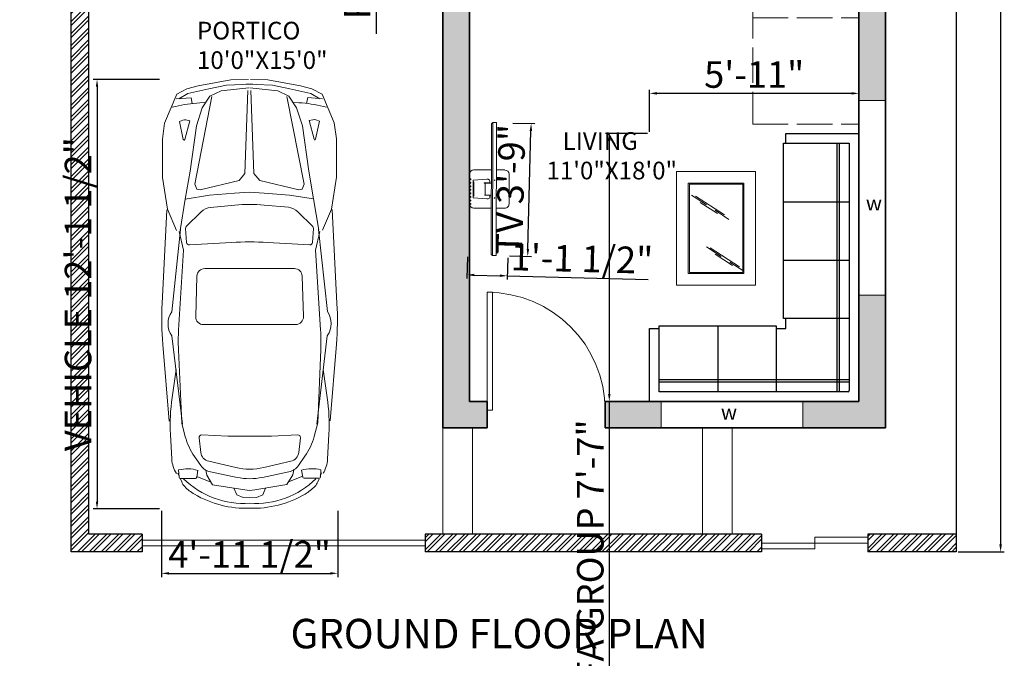
# Model space of a CAD drawing. Units: inches. Extents: x 3488 to 4319, y 780 to 1756.
# Tile 3 of 8: x 3506 to 3839, y 1274 to 1491. Entities that reach past the tile are written whole.
import ezdxf

# ---------------------------------------------------------------- set-up
doc = ezdxf.new("R2010")
doc.units = ezdxf.units.IN
doc.linetypes.add('ACAD_ISO02W100', pattern=[15, 12, -3])
for name, color, linetype, lineweight in [('A-ANNO-IDEN', 7, 'Continuous', 13), ('A-ANNO-TITL', 7, 'Continuous', 25), ('A-AREA-IDEN', 7, 'Continuous', 18), ('A-DOOR', 4, 'Continuous', 18), ('A-EQPM', 8, 'Continuous', 18), ('A-FLOR-OTLN', 7, 'Continuous', 20), ('A-FLOR-STRS-OVHD', 8, 'ACAD_ISO02W100', 18), ('A-WALL', 7, 'Continuous', 35), ('A-WALL-PATT', 252, 'Continuous', 13), ('C-PROP', 7, 'Continuous', 25), ('DIM', 9, 'Continuous', 18), ('FUR', 42, 'Continuous', 18), ('L-FENC', 7, 'Continuous', 30), ('L-FENC-GATE', 4, 'Continuous', 18), ('L-FENC-PATT', 251, 'Continuous', 13), ('L-PKNG-VEHC', 8, 'Continuous', 13), ('window', 130, 'Continuous', 18)]:
    doc.layers.add(name, color=color, linetype=linetype, lineweight=lineweight)
doc.layers.add('TEFRIŞ', color=11, linetype='Continuous')
doc.styles.get("Standard").update_dxf_attribs({"font": 'arial.ttf'})
doc.dimstyles.new('ISO-25', dxfattribs={"dimtxt": 9, "dimasz": 2.5, "dimexe": 1.25, "dimexo": 0.625, "dimtad": 1, "dimdec": 1, "dimlunit": 3, "dimtxsty": 'Standard', "dimcen": 2.5, "dimclrd": 1, "dimclre": 1, "dimclrt": 1, "dimadec": 0, "dimazin": 0, "dimtfac": 1, "dimtdec": 1, "dimtmove": 0, "dimatfit": 3, "dimfxl": 1, "dimarcsym": 0})

# ---------------------------------------------------------------- blocks, each defined once
blk = doc.blocks.new('*U2')
for p, q in [((0, 0), (0, -6)), ((40, 0), (40, -6))]:
    blk.add_line(p, q)
blk.add_lwpolyline([(0, 0), (0, 40), (1.75, 40), (1.75, 0)], close=True)
blk.add_arc((0, 0), 40, 0, 90)
blk = doc.blocks.new('*D6')
at = {"layer": 'Defpoints', "color": 0, "transparency": 16777216}
for p in [(3822.99, 1730.55), (3822.99, 1310.55), (3838.01, 1310.55)]:
    blk.add_point(p, dxfattribs=at)
at = {"layer": 'DIM', "color": 0, "lineweight": -2, "transparency": 16777216}
for p, q in [((3823.61, 1730.55), (3839.26, 1730.55)), ((3838.01, 1728.05), (3838.01, 1313.05)), ((3823.61, 1310.55), (3839.26, 1310.55))]:
    blk.add_line(p, q, dxfattribs=at)
at = {"layer": 'DIM', "color": 0, "transparency": 16777216}
for points in [[(3837.59, 1728.05), (3838.43, 1728.05), (3838.01, 1730.55)], [(3837.59, 1313.05), (3838.43, 1313.05), (3838.01, 1310.55)]]:
    blk.add_solid(points, dxfattribs=at)
at = {"layer": 'DIM', "color": 0, "transparency": 16777216, "insert": (3832.79, 1520.55), "char_height": 9, "attachment_point": 5, "rotation": 90}
blk.add_mtext("35'", dxfattribs=at)
blk = doc.blocks.new('33')
at = {"layer": 'TEFRIŞ'}
for p, q in [((-1013.77, -317.81), (-1013.77, -88.17)), ((-1012.77, -87.17), (-833.45, -87.17)), ((-833.45, -87.17), (-833.45, -150.07)), ((-1005.39, -309.43), (-1005.39, -96.56)), ((-1004.39, -95.56), (-841.84, -95.56)), ((-997, -95.56), (-997, -309.43)), ((-994.9, -95.56), (-994.9, -309.43)), ((-942.48, -152.17), (-942.48, -95.56)), ((-892.16, -152.17), (-892.16, -95.56)), ((-841.84, -95.56), (-841.84, -152.17)), ((-841.84, -103.94), (-1005.39, -103.94)), ((-841.84, -106.04), (-1005.39, -106.04)), ((-950.87, -150.07), (-950.87, -158.46)), ((-942.48, -150.07), (-950.87, -150.07)), ((-841.84, -152.17), (-942.48, -152.17)), ((-833.45, -150.07), (-841.84, -150.07)), ((-1005.39, -158.46), (-948.77, -158.46)), ((-948.77, -158.46), (-948.77, -309.43)), ((-948.77, -208.78), (-1005.39, -208.78)), ((-948.77, -259.1), (-1005.39, -259.1)), ((-948.77, -309.43), (-1005.39, -309.43)), ((-950.87, -309.43), (-950.87, -317.81)), ((-950.87, -317.81), (-1013.77, -317.81))]:
    blk.add_line(p, q, dxfattribs=at)
for centre in [(-1012.77, -88.17), (-1004.39, -96.56)]:
    blk.add_arc(centre, 1, 90, 180, dxfattribs=at)
blk = doc.blocks.new('TV')
at = {"color": 0}
for p, q in [((3967.27, 1784.85), (3967.05, 1784.65)), ((3967.76, 1763.68), (3967.54, 1763.86))]:
    blk.add_line(p, q, dxfattribs=at)
at = {"layer": 'window'}
for p, q in [((3967.54, 1763.86), (3967.05, 1784.65)), ((3964.41, 1777.23), (3967.22, 1777.3)), ((3968.01, 1777.32), (3969.36, 1777.35)), ((3966.53, 1775.82), (3964.33, 1775.61)), ((3964.34, 1775.34), (3964.45, 1775.34)), ((3964.34, 1775.31), (3964.43, 1775.32)), ((3966.14, 1775.2), (3967.01, 1775.22)), ((3966.14, 1775.18), (3967.27, 1775.2)), ((3966.14, 1775.18), (3966.14, 1775.2)), ((3966.3, 1773.29), (3966.26, 1775.18)), ((3964.39, 1773.06), (3964.48, 1773.06)), ((3964.39, 1773.04), (3964.5, 1773.04)), ((3966.61, 1772.66), (3964.4, 1772.77)), ((3966.19, 1773.28), (3967.31, 1773.31)), ((3966.19, 1773.26), (3967.05, 1773.28)), ((3966.19, 1773.26), (3966.19, 1773.28)), ((3964.55, 1771.15), (3967.36, 1771.22)), ((3968.15, 1771.24), (3969.5, 1771.27))]:
    blk.add_line(p, q, dxfattribs=at)
for points in [[(3968.33, 1763.69), (3967.83, 1784.86), (3967.27, 1784.85), (3967.76, 1763.68), (3968.33, 1763.69)], [(3963.86, 1771.81), (3963.75, 1776.54)], [(3964.4, 1772.77), (3964.33, 1775.61)], [(3970.16, 1771.96), (3970.05, 1776.69)], [(3964.48, 1773.06), (3964.43, 1775.32)], [(3964.5, 1773.04), (3964.45, 1775.34)]]:
    blk.add_lwpolyline(points, dxfattribs=at)
for points in [[(3966.53, 1775.82, -0.263666), (3966.93, 1775.69), (3967, 1775.57), (3967.01, 1775.22)], [(3966.61, 1772.66, 0.263666), (3967, 1772.81), (3967.06, 1772.93), (3967.05, 1773.28)]]:
    blk.add_lwpolyline(points, format="xyb", dxfattribs=at)
for centre, radius in [((3963.91, 1775.73), 0.0679), ((3967.77, 1775.68), 0.0451), ((3963.93, 1775.17), 0.0679), ((3963.94, 1774.6), 0.0679), ((3963.95, 1774.04), 0.0679), ((3963.97, 1773.48), 0.0679), ((3963.98, 1772.92), 0.0679), ((3963.99, 1772.35), 0.0679), ((3967.83, 1772.86), 0.0451), ((3964.01, 1771.79), 0.0679)]:
    blk.add_circle(centre, radius, dxfattribs=at)
for centre, start, end in [((3964.42, 1776.56), 91.3414, 181.3414), ((3969.38, 1776.67), 1.3414, 91.3414), ((3964.53, 1771.83), 181.3414, 271.3414), ((3969.49, 1771.94), 271.3414, 1.3414)]:
    blk.add_arc(centre, 0.676, start, end, dxfattribs=at)
blk = doc.blocks.new('A$C4A3239E3')
for p, q in [((1.2507, 1.6335), (2.1522, 1.6799)), ((2.5445, 1.6742), (3.2816, 1.6148)), ((0.1359, 1.4288), (0.1867, 1.515)), ((0.1752, 1.399), (0.1867, 1.5408)), ((0.2661, 1.5794), (0.2592, 1.5495)), ((1.4425, 1.5023), (2.2313, 1.5881)), ((1.4612, 1.5146), (1.6407, 1.4739)), ((1.6407, 1.4739), (2.4076, 1.5225)), ((2.4629, 1.587), (3.3117, 1.4863)), ((2.597, 1.5244), (3.3012, 1.4943)), ((2.7875, 1.5463), (3.0567, 1.5859)), ((3.4104, 1.6024), (3.6491, 1.5899)), ((3.8218, 1.5205), (3.7519, 1.525)), ((3.7813, 1.5317), (3.8128, 1.5185)), ((0.0905, 1.2265), (0.1359, 1.4288)), ((0.3963, 1.4117), (0.388, 1.4492)), ((0.3898, 1.477), (0.4021, 1.5106)), ((0.5758, 1.4596), (0.3963, 1.4117)), ((0.4021, 1.5106), (0.5754, 1.4741)), ((1.4497, 1.5063), (1.149, 1.4553)), ((1.2717, 1.3033), (1.4134, 1.4465)), ((1.4329, 1.4538), (1.567, 1.4437)), ((3.3012, 1.4943), (3.4322, 1.4598)), ((3.8334, 1.3629), (3.8334, 1.5081)), ((3.8376, 1.5081), (3.8668, 1.4958)), ((0.2308, 1.3867), (0.1752, 1.399)), ((1.59, 1.4175), (1.5668, 1.0125)), ((1.8899, 1.3452), (2.2788, 1.3576)), ((3.4434, 1.3284), (3.584, 1.3121)), ((3.6217, 1.372), (3.7108, 1.3099)), ((3.7558, 1.3393), (3.8231, 1.3506)), ((3.8137, 1.3503), (3.8686, 1.2144)), ((0.224, 1.314), (0.2207, 1.2655)), ((1.8186, 0.4085), (1.8178, 1.2708)), ((2.3557, 1.283), (2.3566, 0.3973)), ((3.4158, 1.3024), (3.4294, 1.0516)), ((3.6693, 1.236), (3.7299, 0.9762)), ((3.7535, 1.2644), (3.8014, 1.2553)), ((3.8014, 1.2553), (3.8941, 1.199)), ((0.0565, 1.0588), (0.0905, 1.2265)), ((1.2074, 0.9801), (1.2293, 1.2125)), ((3.7713, 1.2181), (3.8245, 0.9626)), ((3.8941, 1.199), (3.9452, 0.89)), ((0.0481, 0.9038), (0.0565, 1.0588)), ((3.4294, 1.0516), (3.4292, 0.8428)), ((3.9292, 0.9941), (3.9933, 0.9668)), ((3.9933, 0.9668), (4.0172, 0.906)), ((4.0172, 0.906), (4.0211, 0.842)), ((0.0482, 0.7723), (0.0569, 0.6172)), ((3.4299, 0.6309), (3.4292, 0.8396)), ((3.8948, 0.4844), (3.9453, 0.7934)), ((3.9936, 0.7167), (4.0174, 0.7775)), ((4.0174, 0.7775), (4.0211, 0.8416)), ((1.2077, 0.6979), (1.23, 0.4656)), ((1.5911, 0.2613), (1.5671, 0.6662)), ((3.6701, 0.4469), (3.7301, 0.7068)), ((3.772, 0.465), (3.8248, 0.7206)), ((3.9295, 0.6893), (3.9936, 0.7167)), ((0.0569, 0.6172), (0.0912, 0.4496)), ((3.4167, 0.38), (3.4299, 0.6309)), ((3.8022, 0.4279), (3.8948, 0.4844)), ((0.0912, 0.4496), (0.1371, 0.2474)), ((0.2249, 0.3624), (0.2215, 0.4109)), ((3.7543, 0.4187), (3.8022, 0.4279)), ((3.8147, 0.3328), (3.8693, 0.4688)), ((0.2318, 0.2897), (0.1763, 0.2773)), ((1.2726, 0.3749), (1.4146, 0.232)), ((1.8909, 0.3342), (2.2798, 0.3226)), ((3.4444, 0.354), (3.585, 0.3707)), ((3.6228, 0.3107), (3.7117, 0.3731)), ((3.7568, 0.3438), (3.8241, 0.3326)), ((3.8345, 0.3203), (3.8347, 0.1751)), ((0.1371, 0.2474), (0.188, 0.1613)), ((0.1763, 0.2773), (0.1881, 0.1355)), ((0.3975, 0.2651), (0.3892, 0.2275)), ((0.3911, 0.1998), (0.4034, 0.1661)), ((0.5771, 0.2174), (0.3975, 0.2651)), ((0.4034, 0.1661), (0.5767, 0.203)), ((1.451, 0.1722), (1.1502, 0.2226)), ((1.4341, 0.2247), (1.5682, 0.235)), ((1.4625, 0.1639), (1.6419, 0.205)), ((1.6419, 0.205), (2.4089, 0.1579)), ((2.4644, 0.0936), (3.313, 0.1959)), ((3.3024, 0.1879), (3.4334, 0.2226)), ((0.2676, 0.0971), (0.2606, 0.127)), ((1.4438, 0.1762), (2.2328, 0.0919)), ((2.5984, 0.1564), (3.3024, 0.1879)), ((2.7889, 0.1349), (3.0581, 0.0958)), ((3.8231, 0.1627), (3.7532, 0.1581)), ((3.7826, 0.1514), (3.8141, 0.1647)), ((3.8389, 0.1752), (3.8681, 0.1875)), ((1.2522, 0.0446), (2.1538, 0)), ((2.5461, 0.0065), (3.2831, 0.0673)), ((3.4119, 0.0799), (3.6506, 0.0929))]:
    blk.add_line(p, q)
for points in [[(0, 0.8478), (0.0053, 1.0159), (0.0622, 1.3298), (0.0905, 1.4375), (0.1412, 1.5365), (0.4188, 1.6529), (0.572, 1.6743), (0.9399, 1.6743), (1.2458, 1.627), (1.4497, 1.5408)], [(0.0815, 0.8439), (0.1088, 1.11), (0.1609, 1.2182), (0.2737, 1.2906), (0.4463, 1.3472), (0.8811, 1.4091), (1.149, 1.4553), (1.1121, 1.224), (1.0933, 0.9813), (1.085, 0.8389)], [(0.1644, 1.198), (1.0072, 1.3636), (1.0537, 1.3462), (1.0619, 1.3117), (0.9706, 0.937), (0.9035, 0.8818), (0.106, 0.853)], [(0, 0.8281), (0.0056, 0.6601), (0.0632, 0.3462), (0.0916, 0.2386), (0.1426, 0.1398), (0.4204, 0.0239), (0.5737, 0.0028), (0.9415, 0.0032), (1.2473, 0.0511), (1.4511, 0.1377)], [(0.0815, 0.8322), (0.1094, 0.5662), (0.1616, 0.4581), (0.2746, 0.3859), (0.4473, 0.3296), (0.8822, 0.2683), (1.1502, 0.2226), (1.1128, 0.4539), (1.0936, 0.6965), (1.085, 0.8389)], [(0.1651, 0.4782), (1.0082, 0.314), (1.0547, 0.3316), (1.0628, 0.366), (0.9708, 0.7406), (0.9036, 0.7957), (0.1061, 0.8232)]]:
    blk.add_lwpolyline(points)
for centre, radius, start, end in [((2.3053, -1.296), 2.9798, 85.39524, 92.94517), ((2.3463, 1.4226), 0.2016, 54.64918, 124.77695), ((1.7104, 1.2122), 1.4899, 166.91658, 176.08111), ((2.5206, -0.2618), 1.7879, 87.54913, 93.62371), ((3.3168, -0.183), 1.7879, 86.99981, 98.3676), ((3.6355, 1.3122), 0.278, 57.32995, 87.18237), ((4.0973, 1.4394), 0.3558, 166.09608, 196.35351), ((3.821, 1.5081), 0.0124, 0, 86.33043), ((0.4365, 1.46), 0.0497, 159.97873, 192.53841), ((0.5739, 1.4668), 0.00745, 284.96001, 78.11246), ((1.431, 1.429), 0.0248, 85.71507, 135.30465), ((1.5652, 1.4189), 0.0248, 356.72561, 85.71507), ((3.2805, 0.8834), 0.596, 55.07004, 75.25506), ((3.2466, 0.8963), 0.8285, 356.24509, 44.51945), ((3.8091, 1.3584), 0.149, 46.38363, 67.20138), ((3.6181, 1.158), 0.4258, 30.45768, 46.38363), ((1.8923, 1.2708), 0.0745, 91.82012, 179.9989), ((2.2812, 1.2831), 0.0745, 359.92446, 91.82012), ((3.4406, 1.3037), 0.0248, 83.37601, 183.11504), ((3.821, 1.3629), 0.0124, 279.60772, 0), ((3.1325, 0.8724), 0.9892, 358.06945, 30.45768), ((1.3776, 1.1985), 0.149, 135.30465, 174.62136), ((3.5726, 1.2134), 0.0993, 13.12265, 83.37601), ((3.6254, 1.1877), 0.149, 11.76937, 55.07004), ((2.6908, 0.8405), 1.4899, 174.62136, 185.49162), ((4.5417, 0.8423), 2.9798, 176.72561, 183.38736), ((3.1495, 0.8409), 0.596, 346.99033, 13.12265), ((3.2411, 0.841), 0.596, 348.3436, 11.76937), ((1.2382, 0.8392), 1.1919, 176.89416, 183.21881), ((3.6512, 0.8414), 0.298, 350.72464, 9.38834), ((3.2467, 0.7858), 0.8285, 315.59352, 3.86789), ((3.1326, 0.8094), 0.9892, 329.65529, 2.04353), ((1.3783, 0.4799), 0.149, 185.49162, 224.80833), ((1.8931, 0.4086), 0.0745, 180.11408, 268.29286), ((2.2821, 0.397), 0.0745, 268.29286, 0.18852), ((3.4415, 0.3787), 0.0248, 176.99794, 276.73697), ((3.5733, 0.4693), 0.0993, 276.73697, 346.99033), ((3.6261, 0.4951), 0.149, 305.04293, 348.3436), ((1.7111, 0.4671), 1.4899, 184.03187, 193.1964), ((3.2806, 0.7987), 0.596, 284.85791, 305.04293), ((4.0985, 0.2443), 0.3558, 163.75946, 194.01689), ((3.822, 0.3203), 0.0124, 0.11298, 80.50526), ((3.6188, 0.5248), 0.4258, 313.72935, 329.65529), ((0.4377, 0.2169), 0.0497, 167.57457, 200.13424), ((0.5752, 0.2102), 0.00745, 282.00051, 75.15297), ((1.4322, 0.2495), 0.0248, 224.80833, 274.3979), ((1.5663, 0.2598), 0.0248, 274.3979, 3.38736), ((3.8101, 0.3247), 0.149, 292.9116, 313.72935), ((2.5184, 1.9425), 1.7879, 266.48926, 272.56385), ((3.3148, 1.8652), 1.7879, 261.74537, 273.11317), ((3.6364, 0.3706), 0.278, 272.9306, 302.78303), ((3.8223, 0.1751), 0.0124, 273.78255, 0.11298), ((2.3011, 2.9762), 2.9798, 267.1678, 274.71773), ((2.3474, 0.2577), 0.2016, 235.33603, 305.46379)]:
    blk.add_arc(centre, radius, start, end)
blk = doc.blocks.new('GATE-VEHICLE-96IN')
for p, q in [((0, 2), (96, 2)), ((0, 0), (96, 0))]:
    blk.add_line(p, q)
blk = doc.blocks.new('GATE-PEDESTRIAN-36IN')
for p, q in [((18, 4), (36, 4)), ((18, 4), (18, 0)), ((0, 2), (36, 2)), ((0, 0), (18, 0))]:
    blk.add_line(p, q)
blk = doc.blocks.new('STAIR-GROUND-OVERHEAD-FLIGHT')
for p, q in [((0, 86), (0, 0)), ((0, 86), (36, 86)), ((0, 76), (36, 76)), ((0, 66), (36, 66)), ((0, 56), (36, 56)), ((0, 46), (36, 46)), ((0, 36), (36, 36)), ((0, 0), (36, 0))]:
    blk.add_line(p, q)
blk = doc.blocks.new('*D90')
at = {"layer": 'Defpoints', "color": 0, "transparency": 16777216}
for p in [(3630.4, 1643.52), (3626.38, 1616.73), (3630.4, 1616.73)]:
    blk.add_point(p, dxfattribs=at)
at = {"layer": 'DIM', "color": 1, "lineweight": -2, "transparency": 16777216}
for p, q in [((3629.78, 1643.52), (3625.13, 1643.52)), ((3626.38, 1641.02), (3626.38, 1619.23)), ((3629.78, 1616.73), (3625.13, 1616.73)), ((3626.38, 1616.73), (3626.38, 1486.14))]:
    blk.add_line(p, q, dxfattribs=at)
at = {"layer": 'DIM', "color": 1, "transparency": 16777216}
for points in [[(3625.97, 1641.02), (3626.8, 1641.02), (3626.38, 1643.52)], [(3625.97, 1619.23), (3626.8, 1619.23), (3626.38, 1616.73)]]:
    blk.add_solid(points, dxfattribs=at)
at = {"layer": 'DIM', "color": 1, "transparency": 16777216, "insert": (3621.1, 1550.18), "char_height": 9, "attachment_point": 5, "rotation": 90}
blk.add_mtext('REFRIGERATOR 2\'-3"', dxfattribs=at)
blk = doc.blocks.new('*D102')
at = {"layer": 'Defpoints', "color": 0, "transparency": 16777216}
for p in [(3719, 1452.36), (3705.37, 1361.55), (3719, 1361.55)]:
    blk.add_point(p, dxfattribs=at)
at = {"layer": 'DIM', "color": 1, "lineweight": -2, "transparency": 16777216}
for p, q in [((3718.37, 1452.36), (3704.12, 1452.36)), ((3705.37, 1449.86), (3705.37, 1364.05)), ((3718.37, 1361.55), (3704.12, 1361.55)), ((3705.37, 1361.55), (3705.37, 1246.6))]:
    blk.add_line(p, q, dxfattribs=at)
at = {"layer": 'DIM', "color": 1, "transparency": 16777216}
for points in [[(3704.96, 1449.86), (3705.79, 1449.86), (3705.37, 1452.36)], [(3704.96, 1364.05), (3705.79, 1364.05), (3705.37, 1361.55)]]:
    blk.add_solid(points, dxfattribs=at)
at = {"layer": 'DIM', "color": 1, "transparency": 16777216, "insert": (3700.09, 1302.83), "char_height": 9, "attachment_point": 5, "rotation": 90}
blk.add_mtext('SOFA GROUP 7\'-7"', dxfattribs=at)
blk = doc.blocks.new('*D103')
at = {"layer": 'Defpoints', "color": 0, "transparency": 16777216}
for p in [(3719, 1465.98), (3719, 1452.36), (3789.99, 1452.36)]:
    blk.add_point(p, dxfattribs=at)
at = {"layer": 'DIM', "color": 1, "lineweight": -2, "transparency": 16777216}
for p, q in [((3719, 1452.98), (3719, 1467.23)), ((3787.49, 1465.98), (3721.5, 1465.98)), ((3789.99, 1452.98), (3789.99, 1467.23))]:
    blk.add_line(p, q, dxfattribs=at)
at = {"layer": 'DIM', "color": 1, "transparency": 16777216}
for points in [[(3721.5, 1466.4), (3721.5, 1465.56), (3719, 1465.98)], [(3787.49, 1466.4), (3787.49, 1465.56), (3789.99, 1465.98)]]:
    blk.add_solid(points, dxfattribs=at)
at = {"layer": 'DIM', "color": 1, "transparency": 16777216, "insert": (3754.49, 1471.2), "char_height": 9, "attachment_point": 5}
blk.add_mtext('5\'-11"', dxfattribs=at)
blk = doc.blocks.new('*D104')
at = {"layer": 'Defpoints', "color": 0, "transparency": 16777216}
for p in [(3672.11, 1455.94), (3678.87, 1455.77), (3670.96, 1410.88)]:
    blk.add_point(p, dxfattribs=at)
at = {"layer": 'DIM', "color": 1, "lineweight": -2, "transparency": 16777216}
for p, q in [((3672.73, 1455.92), (3680.12, 1455.73)), ((3677.78, 1413.2), (3678.8, 1453.27)), ((3671.59, 1410.86), (3678.97, 1410.67))]:
    blk.add_line(p, q, dxfattribs=at)
at = {"layer": 'DIM', "color": 1, "transparency": 16777216}
for points in [[(3678.39, 1453.28), (3679.22, 1453.26), (3678.87, 1455.77)], [(3677.37, 1413.22), (3678.2, 1413.19), (3677.72, 1410.71)]]:
    blk.add_solid(points, dxfattribs=at)
at = {"layer": 'DIM', "color": 1, "transparency": 16777216, "insert": (3673.07, 1433.37), "char_height": 9, "attachment_point": 5, "rotation": 88.5431}
blk.add_mtext('TV 3\'-9"', dxfattribs=at)
blk = doc.blocks.new('*D105')
at = {"layer": 'Defpoints', "color": 0, "transparency": 16777216}
for p in [(3657.29, 1411.23), (3670.96, 1410.88), (3670.79, 1404.12)]:
    blk.add_point(p, dxfattribs=at)
at = {"layer": 'DIM', "color": 1, "lineweight": -2, "transparency": 16777216}
for p, q in [((3657.28, 1410.6), (3657.09, 1403.22)), ((3670.95, 1410.25), (3670.76, 1402.87)), ((3659.62, 1404.4), (3668.29, 1404.18)), ((3670.79, 1404.12), (3718.57, 1402.9))]:
    blk.add_line(p, q, dxfattribs=at)
at = {"layer": 'DIM', "color": 1, "transparency": 16777216}
for points in [[(3659.63, 1404.82), (3659.61, 1403.99), (3657.12, 1404.47)], [(3668.3, 1404.6), (3668.28, 1403.77), (3670.79, 1404.12)]]:
    blk.add_solid(points, dxfattribs=at)
at = {"layer": 'DIM', "color": 1, "transparency": 16777216, "insert": (3696.06, 1408.76), "char_height": 9, "attachment_point": 5, "rotation": 358.5431}
blk.add_mtext('1\'-1 1/2"', dxfattribs=at)
blk = doc.blocks.new('*D106')
at = {"layer": 'Defpoints', "color": 0, "transparency": 16777216}
for p in [(3553.59, 1470.72), (3531.74, 1325.11), (3553.59, 1325.11)]:
    blk.add_point(p, dxfattribs=at)
at = {"layer": 'DIM', "color": 1, "lineweight": -2, "transparency": 16777216}
for p, q in [((3552.96, 1470.72), (3530.49, 1470.72)), ((3531.74, 1468.22), (3531.74, 1327.61)), ((3552.96, 1325.11), (3530.49, 1325.11))]:
    blk.add_line(p, q, dxfattribs=at)
at = {"layer": 'DIM', "color": 1, "transparency": 16777216}
for points in [[(3531.33, 1468.22), (3532.16, 1468.22), (3531.74, 1470.72)], [(3531.33, 1327.61), (3532.16, 1327.61), (3531.74, 1325.11)]]:
    blk.add_solid(points, dxfattribs=at)
at = {"layer": 'DIM', "color": 1, "transparency": 16777216, "insert": (3526.47, 1397.92), "char_height": 9, "attachment_point": 5, "rotation": 90}
blk.add_mtext('VEHICLE 12\'-1 1/2"', dxfattribs=at)
blk = doc.blocks.new('*D107')
at = {"layer": 'Defpoints', "color": 0, "transparency": 16777216}
for p in [(3553.59, 1325.11), (3613.31, 1325.11), (3613.31, 1303.27)]:
    blk.add_point(p, dxfattribs=at)
at = {"layer": 'DIM', "color": 1, "lineweight": -2, "transparency": 16777216}
for p, q in [((3553.59, 1324.49), (3553.59, 1302.02)), ((3613.31, 1324.49), (3613.31, 1302.02)), ((3556.09, 1303.27), (3610.81, 1303.27))]:
    blk.add_line(p, q, dxfattribs=at)
at = {"layer": 'DIM', "color": 1, "transparency": 16777216}
for points in [[(3556.09, 1303.69), (3556.09, 1302.85), (3553.59, 1303.27)], [(3610.81, 1303.69), (3610.81, 1302.85), (3613.31, 1303.27)]]:
    blk.add_solid(points, dxfattribs=at)
at = {"layer": 'DIM', "color": 1, "transparency": 16777216, "insert": (3583.45, 1308.55), "char_height": 9, "attachment_point": 5}
blk.add_mtext('4\'-11 1/2"', dxfattribs=at)

msp = doc.modelspace()

# ---------------------------------------------------------------- hatches: boundary and pattern name
at = {"layer": 'A-WALL-PATT', "transparency": 33554687}
h = msp.add_hatch(color=256, dxfattribs=at)
h.dxf.hatch_style = 1
h.paths.add_polyline_path([(3657.99, 1505.55), (3657.99, 1535.55), (3651.99, 1535.55), (3651.99, 1505.55), (3609.99, 1505.55), (3609.99, 1544.55), (3603.99, 1544.55), (3603.99, 1505.55), (3555.99, 1505.55), (3555.99, 1514.55), (3546.99, 1514.55), (3546.99, 1496.55), (3648.99, 1496.55), (3648.99, 1352.55), (3663.99, 1352.55), (3663.99, 1361.55), (3657.99, 1361.55)])
h.paths.add_polyline_path([(3722.99, 1361.55), (3719, 1361.55), (3703.99, 1361.55), (3703.99, 1352.55), (3722.99, 1352.55)])
h.paths.add_polyline_path([(3798.99, 1397.55), (3789.99, 1397.55), (3789.99, 1361.95), (3789.99, 1361.55), (3770.99, 1361.55), (3770.99, 1352.55), (3798.99, 1352.55)])
h.paths.add_polyline_path([(3798.99, 1547.58), (3789.99, 1547.58), (3789.99, 1463.55), (3798.99, 1463.55)])
h.paths.add_polyline_path([(3798.99, 1613.55), (3789.99, 1613.55), (3789.99, 1583.55), (3693.99, 1583.55), (3693.99, 1577.55), (3789.99, 1577.55), (3789.99, 1571.58), (3798.99, 1571.58)])
h.paths.add_polyline_path([(3798.99, 1712.55), (3717.99, 1712.55), (3717.99, 1703.55), (3789.99, 1703.55), (3789.99, 1673.55), (3798.99, 1673.55)])
h.paths.add_polyline_path([(3681.99, 1712.55), (3627.99, 1712.55), (3627.99, 1703.55), (3651.99, 1703.55), (3651.99, 1577.55), (3657.99, 1577.55), (3657.99, 1703.55), (3681.99, 1703.55)])
h.paths.add_polyline_path([(3591.99, 1712.55), (3546.99, 1712.55), (3546.99, 1667.55), (3555.99, 1667.55), (3555.99, 1703.55), (3591.99, 1703.55)])
edge = h.paths.add_edge_path()
edge.add_line((3555.99, 1619.55), (3546.99, 1619.55))
edge.add_line((3546.99, 1619.55), (3546.99, 1538.55))
edge.add_line((3546.99, 1538.55), (3555.99, 1538.55))
edge.add_line((3555.99, 1538.55), (3555.99, 1565.03))
edge.add_ellipse((3556.27, 1565.11), major_axis=(0.21, 0.21), ratio=0.999043, start_angle=135, end_angle=151.1563, ccw=False)
edge.add_line((3555.98, 1565.08), (3555.99, 1577.26))
edge.add_line((3555.99, 1577.26), (3555.99, 1577.55))
edge.add_line((3555.99, 1577.55), (3603.99, 1577.55))
edge.add_line((3603.99, 1577.55), (3603.99, 1574.55))
edge.add_line((3603.99, 1574.55), (3609.99, 1574.55))
edge.add_line((3609.99, 1574.55), (3609.99, 1583.55))
edge.add_line((3609.99, 1583.55), (3555.99, 1583.55))
edge.add_line((3555.99, 1583.55), (3555.99, 1619.55))
at = {"layer": 'L-FENC-PATT', "transparency": 33554687}
h = msp.add_hatch(dxfattribs=at)
h.set_pattern_fill('ANSI32', color=256, scale=0.3)
h.paths.add_polyline_path([(3546.99, 1505.55), (3522.99, 1505.55), (3522.99, 1310.55), (3546.99, 1310.55), (3546.99, 1316.55), (3528.99, 1316.55), (3528.99, 1496.55), (3546.99, 1496.55)])
h.paths.add_polyline_path([(3756.99, 1316.55), (3642.99, 1316.55), (3642.99, 1310.55), (3756.99, 1310.55)])
h.paths.add_polyline_path([(3822.99, 1316.55), (3792.99, 1316.55), (3792.99, 1310.55), (3822.99, 1310.55)])

# ---------------------------------------------------------------- linework, layer by layer
at = {"layer": 'A-FLOR-OTLN'}
for p, q in [((3648.99, 1352.55), (3648.99, 1316.55)), ((3658.99, 1352.55), (3658.99, 1316.55)), ((3736.99, 1352.55), (3736.99, 1316.55)), ((3746.99, 1352.55), (3746.99, 1316.55))]:
    msp.add_line(p, q, dxfattribs=at)
at = {"layer": 'A-WALL'}
for p, q in [((3798.99, 1712.55), (3798.99, 1352.55)), ((3789.99, 1577.55), (3789.99, 1361.55)), ((3657.99, 1505.55), (3657.99, 1361.55)), ((3648.99, 1496.55), (3648.99, 1352.55)), ((3657.99, 1361.55), (3663.99, 1361.55)), ((3663.99, 1361.55), (3663.99, 1352.55)), ((3703.99, 1361.55), (3703.99, 1352.55)), ((3703.99, 1361.55), (3789.99, 1361.55)), ((3648.99, 1352.55), (3663.99, 1352.55)), ((3703.99, 1352.55), (3798.99, 1352.55))]:
    msp.add_line(p, q, dxfattribs=at)
at = {"layer": 'C-PROP'}
for p, q in [((3522.99, 1310.55), (3522.99, 1730.55)), ((3822.99, 1730.55), (3822.99, 1310.55))]:
    msp.add_line(p, q, dxfattribs=at)
at = {"layer": 'FUR'}
for p, q in [((3728.2, 1400.98), (3728.2, 1439.49)), ((3728.2, 1439.49), (3754.94, 1439.49)), ((3754.94, 1439.49), (3754.94, 1400.98)), ((3732.13, 1404.92), (3732.13, 1435.55)), ((3732.13, 1435.55), (3751, 1435.55)), ((3732.53, 1405.31), (3732.53, 1435.15)), ((3732.53, 1435.15), (3750.61, 1435.15)), ((3750.61, 1435.15), (3750.61, 1405.31)), ((3751, 1435.55), (3751, 1404.92)), ((3738.29, 1428.24), (3733.23, 1431.52)), ((3744.41, 1424.76), (3734.54, 1431.17)), ((3742.04, 1425.22), (3736.19, 1429.02)), ((3745.94, 1423.27), (3741.21, 1426.34)), ((3743.32, 1410.7), (3738.27, 1413.98)), ((3749.45, 1407.22), (3739.58, 1413.62)), ((3747.08, 1407.68), (3741.22, 1411.48)), ((3750.98, 1405.73), (3746.24, 1408.8)), ((3750.61, 1405.31), (3732.53, 1405.31)), ((3751, 1404.92), (3732.13, 1404.92)), ((3754.94, 1400.98), (3728.2, 1400.98))]:
    msp.add_line(p, q, dxfattribs=at)
at = {"layer": 'L-FENC'}
for p, q in [((3528.99, 1316.55), (3528.99, 1496.55)), ((3546.99, 1316.55), (3528.99, 1316.55)), ((3546.99, 1316.55), (3546.99, 1310.55)), ((3642.99, 1316.55), (3642.99, 1310.55)), ((3756.99, 1316.55), (3642.99, 1316.55)), ((3756.99, 1316.55), (3756.99, 1310.55)), ((3822.99, 1316.55), (3792.99, 1316.55)), ((3792.99, 1316.55), (3792.99, 1310.55)), ((3546.99, 1310.55), (3522.99, 1310.55)), ((3756.99, 1310.55), (3642.99, 1310.55)), ((3822.99, 1310.55), (3792.99, 1310.55))]:
    msp.add_line(p, q, dxfattribs=at)
at = {"layer": 'window'}
for p, q in [((3789.99, 1463.55), (3798.99, 1463.55)), ((3789.99, 1397.55), (3798.99, 1397.55)), ((3722.99, 1361.55), (3722.99, 1352.55)), ((3770.99, 1361.55), (3770.99, 1352.55))]:
    msp.add_line(p, q, dxfattribs=at)

# ---------------------------------------------------------------- block references
at = {"layer": 'A-DOOR'}
msp.add_blockref('*U2', (3663.99, 1358.55), dxfattribs=at)
at = {"layer": 'A-EQPM', "xscale": 2.127748957344282, "yscale": 2.127748957344282, "zscale": 2.127748957344282, "rotation": 358.5430845181614}
msp.add_blockref('TV', (-4869.24, -2125.79), dxfattribs=at)
at = {"layer": 'A-FLOR-STRS-OVHD'}
msp.add_blockref('STAIR-GROUND-OVERHEAD-FLIGHT', (3753.99, 1455.55), dxfattribs=at)
at = {"layer": 'FUR', "xscale": 0.393701, "yscale": 0.393701, "zscale": 0.393701, "rotation": 180}
msp.add_blockref('33', (3390.87, 1327.23), dxfattribs=at)
at = {"layer": 'L-FENC-GATE'}
for name, p in [('GATE-PEDESTRIAN-36IN', (3756.99, 1311.55)), ('GATE-VEHICLE-96IN', (3546.99, 1312.55))]:
    msp.add_blockref(name, p, dxfattribs=at)
at = {"layer": 'L-PKNG-VEHC', "xscale": 35.27598425228, "yscale": 35.27598425228, "zscale": 35.27598425228, "rotation": 270}
msp.add_blockref('A$C4A3239E3', (3553.82, 1470.72), dxfattribs=at)

# ---------------------------------------------------------------- texts
at = {"layer": 'A-ANNO-IDEN'}
for p in [(3792.33, 1426.29), (3743.2, 1355.39)]:
    msp.add_text('w', height=5, dxfattribs=at).set_placement(p)
at = {"layer": 'A-ANNO-TITL', "insert": (3597.32, 1287.85), "char_height": 10, "attachment_point": 1}
msp.add_mtext_dynamic_manual_height_columns('GROUND FLOOR PLAN', width=202.5735, gutter_width=25, heights=[0], dxfattribs=at)
at = {"layer": 'A-AREA-IDEN', "char_height": 6, "attachment_point": 1}
for s, insert in [('PORTICO\\P10\'0"X15\'0"', (3565.61, 1490.25)), ('   LIVING\\P11\'0"X18\'0"', (3684.07, 1452.82))]:
    msp.add_mtext_dynamic_manual_height_columns(s, width=83.4163, gutter_width=25, heights=[0], dxfattribs=dict(at, insert=insert))

# ---------------------------------------------------------------- dimensions: what is measured, and where the dimension line sits
at = {"layer": 'DIM'}
for base, p1, p2, angle, override, picture, middle in [((3838.01, 1310.55), (3822.99, 1730.55), (3822.99, 1310.55), 90, {"dimclrd": 0, "dimclre": 0, "dimclrt": 0}, '*D6', (3832.79, 1520.55)), ((3719, 1465.98), (3789.99, 1452.36), (3719, 1452.36), 180, {"dimdec": 1, "dimlfac": 1, "dimrnd": 0, "dimzin": 1, "dimdsep": 46, "dimlunit": 4, "dimfrac": 2}, '*D103', (3754.49, 1471.2)), ((3670.79, 1404.12), (3657.29, 1411.23), (3670.96, 1410.88), 358.5431, {"dimdec": 1, "dimlfac": 1, "dimrnd": 0, "dimzin": 1, "dimdsep": 46, "dimlunit": 4, "dimfrac": 2}, '*D105', (3696.06, 1408.76))]:
    dim = msp.add_linear_dim(base=base, p1=p1, p2=p2, angle=angle, dimstyle='ISO-25', override=override, dxfattribs=at)
    dim.commit()
    dim.dimension.update_dxf_attribs({"geometry": picture, "text_midpoint": middle})
for base, p1, p2, angle, text, picture, middle in [((3626.38, 1616.73), (3630.4, 1643.52), (3630.4, 1616.73), 270, 'REFRIGERATOR <>', '*D90', (3621.1, 1550.18)), ((3531.74, 1325.11), (3553.59, 1470.72), (3553.59, 1325.11), 270, 'VEHICLE <>', '*D106', (3526.47, 1397.92)), ((3678.87, 1455.77), (3670.96, 1410.88), (3672.11, 1455.94), 88.5431, 'TV <>', '*D104', (3673.07, 1433.37)), ((3705.37, 1361.55), (3719, 1452.36), (3719, 1361.55), 270, 'SOFA GROUP <>', '*D102', (3700.09, 1302.83))]:
    dim = msp.add_linear_dim(base=base, p1=p1, p2=p2, angle=angle, text=text, dimstyle='ISO-25', override={"dimdec": 1, "dimlfac": 1, "dimrnd": 0, "dimzin": 1, "dimdsep": 46, "dimlunit": 4, "dimfrac": 2}, dxfattribs=at)
    dim.commit()
    dim.dimension.update_dxf_attribs({"geometry": picture, "text_midpoint": middle})
dim = msp.add_linear_dim(base=(3613.31, 1303.27), p1=(3553.59, 1325.11), p2=(3613.31, 1325.11), dimstyle='ISO-25', override={"dimdec": 1, "dimlfac": 1, "dimrnd": 0, "dimzin": 1, "dimdsep": 46, "dimlunit": 4, "dimfrac": 2}, dxfattribs=at)
dim.commit()
dim.dimension.update_dxf_attribs({"geometry": '*D107', "text_midpoint": (3583.45, 1308.55)})

doc.saveas('drawing.dxf')
